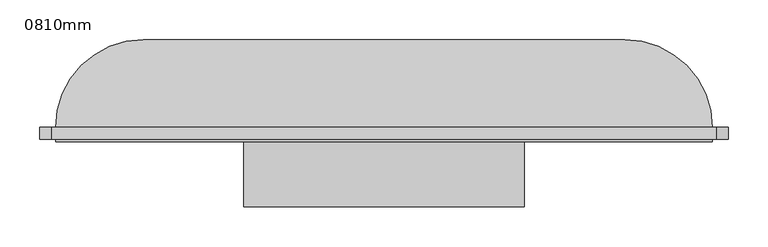
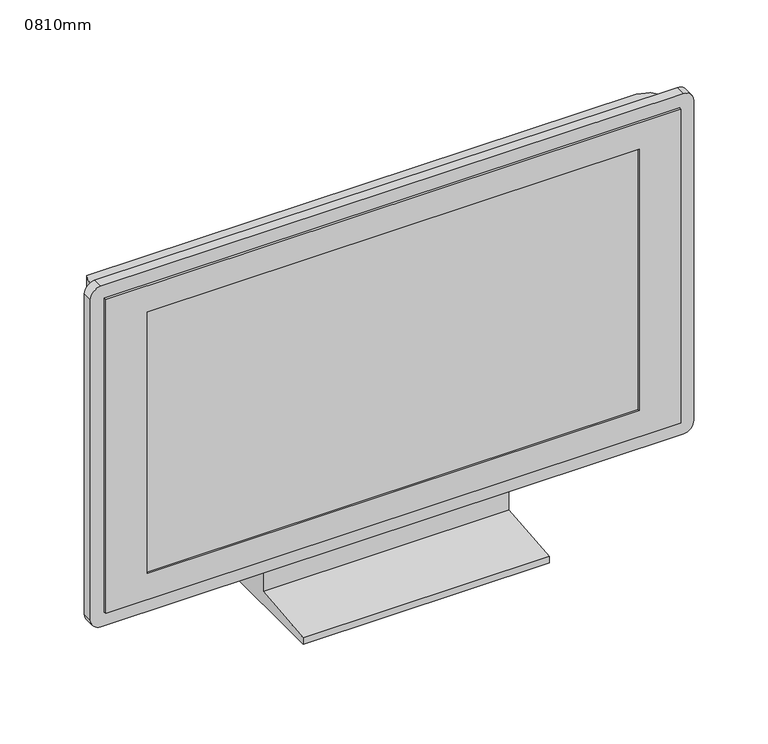
"""IFC4 building model written with IfcOpenShell, lengths in millimetres: furniture geometry, 0810mm."""

from ifc_helpers import new_model, si_unit, point, frame, frame_2d, origin, place, context, project, spatial, polyline, circle_curve, ellipse_curve, trimmed, segment, composite_curve, outline, extrude, faceted_brep, source, transform, mapped, element, save
from ifc_brep_helpers import plane_surface, cylinder_surface, advanced_brep


def furniture_0810mm_51289c3c(model_context):
    return source(origin(), model_context, "Body", "SolidModel", [
        advanced_brep(
        [(-416.9248214, -51.4613764, 80.0), (409.0357931, -51.4613764, 80.0), (409.0357931, -51.4613764, 557.1392838), (-416.9248214, -51.4613764, 557.1392838), (299.0357931, 58.5386236, 80.0), (-306.9248214, 58.5386236, 80.0), (-306.9248214, 58.5386236, 447.1392838), (299.0357931, 58.5386236, 447.1392838)],
        [
            (0, 1),
            (1, 2),
            (2, 3),
            (3, 0),
            (4, 5),
            (5, 6),
            (6, 7),
            (7, 4),
            (0, 5, circle_curve(frame((-306.9248214, -51.4613764, 80.0), z_axis=(0.0, 0.0, -1.0), x_axis=(-1.0, 0.0, 0.0)), 110.0)),
            (4, 1, circle_curve(frame((299.0357931, -51.4613764, 80.0), z_axis=(0.0, 0.0, -1.0), x_axis=(1.0, 0.0, 0.0)), 110.0)),
            (7, 2, ellipse_curve(frame((299.0357931, -51.4613764, 447.1392838), z_axis=(0.7071067811865475, 0.0, -0.7071067811865475), x_axis=(0.7071067811865474, 0.0, 0.7071067811865476)), 155.5634919, 110.0)),
            (6, 3, ellipse_curve(frame((-306.9248214, -51.4613764, 447.1392838), z_axis=(0.7071067811865475, 0.0, 0.7071067811865475), x_axis=(-0.7071067811865476, 0.0, 0.7071067811865474)), 155.5634919, 110.0)),
        ],
        [
            plane_surface(frame((-416.9248214, -51.4613764, 557.1392838), z_axis=(0.0, -1.0, 0.0), x_axis=(-1.0, 0.0, 0.0))),
            plane_surface(frame((-416.9248214, 58.5386236, 557.1392838), z_axis=(0.0, 1.0, 0.0), x_axis=(1.0, 0.0, 0.0))),
            plane_surface(frame((-416.9248214, -51.4613764, 80.0), z_axis=(0.0, 0.0, -1.0), x_axis=(0.0, 1.0, 0.0))),
            cylinder_surface(frame((299.0357931, -51.4613764, 80.0), z_axis=(0.0, 0.0, 1.0), x_axis=(1.0, 0.0, 0.0)), 110.0),
            cylinder_surface(frame((409.0357931, -51.4613764, 447.1392838), z_axis=(-1.0, 0.0, 0.0), x_axis=(0.0, 0.0, 1.0)), 110.0),
            cylinder_surface(frame((-306.9248214, -51.4613764, 557.1392838), z_axis=(0.0, 0.0, -1.0), x_axis=(-1.0, 0.0, 0.0)), 110.0),
        ],
        [
            (0, [[1, 2, 3, 4]]),
            (1, [[5, 6, 7, 8]]),
            (2, [[-1, 9, -5, 10]]),
            (3, [[11, -2, -10, -8]]),
            (4, [[-11, -7, 12, -3]]),
            (5, [[-12, -6, -9, -4]]),
        ],
    ),
        extrude(outline(composite_curve([segment(polyline([(577.1392838, 414.0357931), (577.1392838, -421.9248214)]), True, "CONTINUOUS"), segment(trimmed(circle_curve(frame_2d((562.1392838, -421.9248214)), 15.0), [point((577.1392838, -421.9248214))], [point((562.1392838, -436.9248214))], False, "CARTESIAN"), True, "CONTINUOUS"), segment(polyline([(562.1392838, -436.9248214), (75.0, -436.9248214)]), True, "CONTINUOUS"), segment(trimmed(circle_curve(frame_2d((75.0, -421.9248214)), 15.0), [point((75.0, -436.9248214))], [point((60.0, -421.9248214))], False, "CARTESIAN"), True, "CONTINUOUS"), segment(polyline([(60.0, -421.9248214), (60.0, 414.0357931)]), True, "CONTINUOUS"), segment(trimmed(circle_curve(frame_2d((75.0, 414.0357931)), 15.0), [point((60.0, 414.0357931))], [point((75.0, 429.0357931))], False, "CARTESIAN"), True, "CONTINUOUS"), segment(polyline([(75.0, 429.0357931), (562.1392838, 429.0357931)]), True, "CONTINUOUS"), segment(trimmed(circle_curve(frame_2d((562.1392838, 414.0357931)), 15.0), [point((562.1392838, 429.0357931))], [point((577.1392838, 414.0357931))], False, "CARTESIAN"), True, "CONTINUOUS")], self_intersect=False), holes=[polyline([(557.1392838, 409.0357931), (80.0, 409.0357931), (80.0, -416.9248214), (557.1392838, -416.9248214), (557.1392838, 409.0357931)])]), frame((0.0, -66.4613764, 0.0), z_axis=(0.0, 1.0, 0.0), x_axis=(0.0, 0.0, 1.0)), (0.0, 0.0, 1.0), 15.0),
        faceted_brep([(409.0357931, -69.4613764, 557.1392838), (-416.9248214, -69.4613764, 557.1392838), (-416.9248214, -69.4613764, 80.0), (409.0357931, -69.4613764, 80.0), (-356.9248214, -69.4613764, 517.1392838), (349.0357931, -69.4613764, 517.1392838), (349.0357931, -69.4613764, 120.0), (-356.9248214, -69.4613764, 120.0), (409.0357931, -51.4613764, 557.1392838), (409.0357931, -51.4613764, 80.0), (-416.9248214, -51.4613764, 80.0), (-416.9248214, -51.4613764, 557.1392838), (-356.9248214, -66.4613764, 517.1392838), (-356.9248214, -66.4613764, 120.0), (349.0357931, -66.4613764, 120.0), (349.0357931, -66.4613764, 517.1392838)], [[[0, 1, 2, 3], [4, 5, 6, 7]], [[8, 9, 10, 11]], [[1, 0, 8, 11]], [[2, 1, 11, 10]], [[3, 2, 10, 9]], [[0, 3, 9, 8]], [[12, 13, 14, 15]], [[12, 15, 5, 4]], [[15, 14, 6, 5]], [[14, 13, 7, 6]], [[13, 12, 4, 7]]]),
        extrude(outline(polyline([(-51.4613764, 80.0), (-1.4613764, 80.0), (48.5386236, 0.0), (-151.4613764, 0.0), (-151.4613764, 10.0), (-51.4613764, 20.0), (-51.4613764, 80.0)])), frame((-180.4346678, 0.0, 0.0), z_axis=(1.0, 0.0, 0.0), x_axis=(0.0, 1.0, 0.0)), (0.0, 0.0, 1.0), 352.9803073),
    ])


if __name__ == "__main__":
    model = new_model("IFC4")
    model_context = context("Model", 3, world=origin())
    ifc_project = project(units=[si_unit("LENGTHUNIT", "METRE", prefix="MILLI")], contexts=[model_context])
    site = spatial("IfcSite", under=ifc_project)
    building = spatial("IfcBuilding", under=site)
    placement = place(None, origin())
    furniture_0810mm_shape = furniture_0810mm_51289c3c(model_context)
    element("IfcFurniture", 1, ObjectType="0810mm", at=placement, inside=building, context=model_context, shape_type="MappedRepresentation", body=[
        mapped(furniture_0810mm_shape, transform((0.0, 0.0, 0.0), x_axis=(1.0, 0.0, 0.0), y_axis=(0.0, 1.0, 0.0), z_axis=(0.0, 0.0, 1.0))),
    ])
    save(model, "model.ifc")

# Revit data of these elements
# Type "0810mm"
#   SinAng = 0.49 mm
#   L = 705.961 mm
#   H = 397.139 mm
#   Thickness = 110 mm
#   Diagonal = 810 mm
#   CosAng = 0.872 mm
#   Stand [instance default] = yes
#   Default Elevation = 0
# Element 1 (IfcFurniture, "0810mm")
#   Materials on its faces: "TV - Black", "TV - Glass", "TV - Screen"
# Materials
#   "TV - Black": colour RGB 49 49 49, transparency 0
#   "TV - Glass": colour RGB 157 157 157, transparency 0.9
#   "TV - Screen": colour RGB 0 0 0, transparency 0
